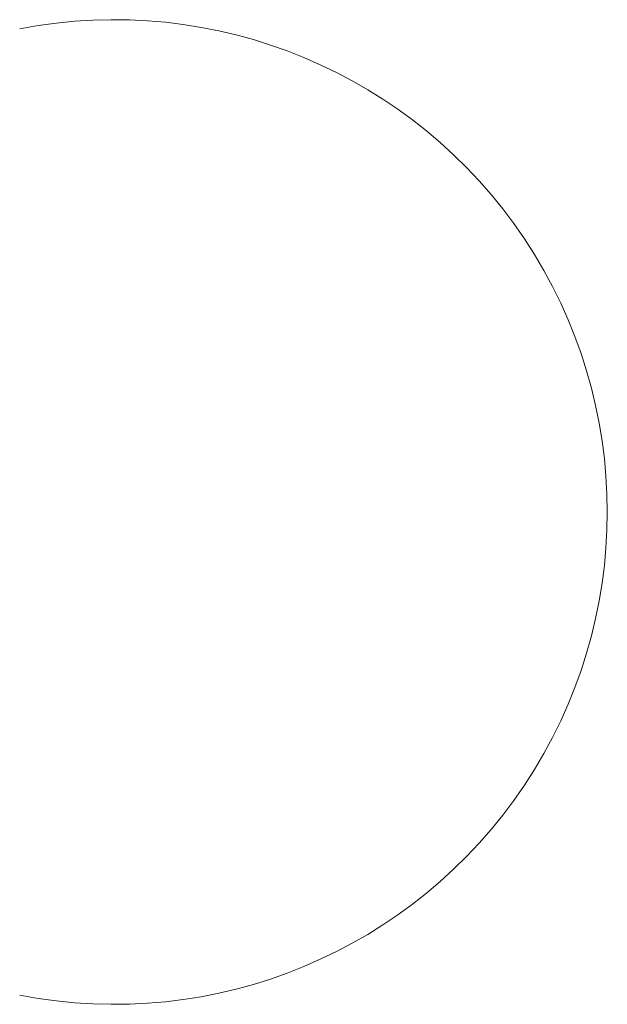
# Model space of a CAD drawing. Units: millimetres. Extents: x 1901.5 to 1919.4, y 750.1 to 780.1.
import ezdxf

# ---------------------------------------------------------------- set-up
doc = ezdxf.new("R2010")
doc.units = ezdxf.units.MM
doc.layers.add('M-CONS', color=8, linetype='Continuous', lineweight=13)

msp = doc.modelspace()

# ---------------------------------------------------------------- linework, layer by layer
at = {"layer": 'M-CONS'}
msp.add_arc((1904.365, 765.129), 15, 258.9125, 101.0875, dxfattribs=at)

doc.saveas('drawing.dxf')
